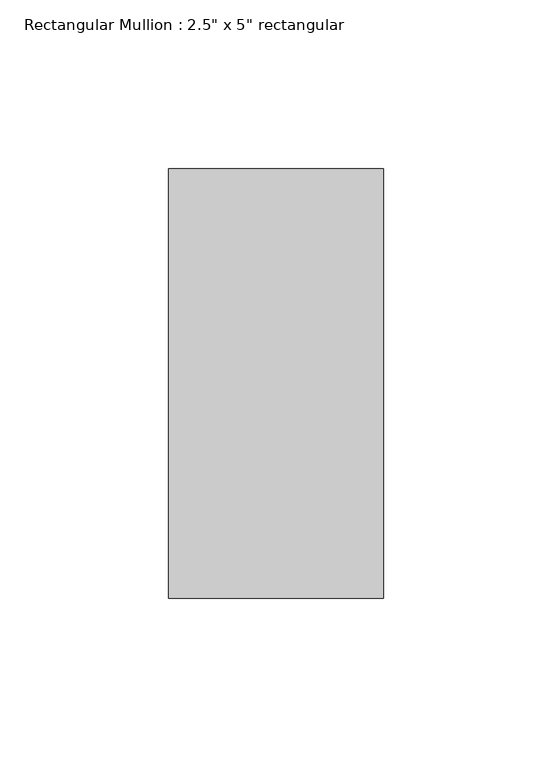
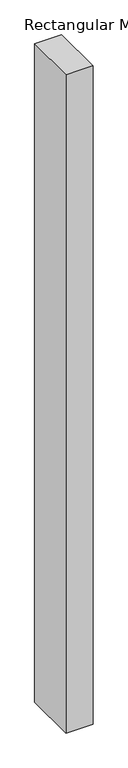
"""IFC4 building model written with IfcOpenShell, lengths in millimetres: member geometry."""

from ifc_helpers import new_model, si_unit, frame, origin, place, context, project, spatial, polyline, outline, extrude, source, transform, mapped, element, save


def member_ce46b7cd(model_context):
    return source(origin(), model_context, "Body", "SweptSolid", [
        extrude(outline(polyline([(0.0, 63.5), (0.0, -63.5), (-63.5, -63.5), (-63.5, 63.5), (0.0, 63.5)])), frame((0.0, 0.0, -1633.9367938), z_axis=(0.0, 0.0, 1.0), x_axis=(1.0, 0.0, 0.0)), (0.0, 0.0, 1.0), 1633.9367938),
    ])


if __name__ == "__main__":
    model = new_model("IFC4")
    model_context = context("Model", 3, world=origin())
    ifc_project = project(units=[si_unit("LENGTHUNIT", "METRE", prefix="MILLI")], contexts=[model_context])
    site = spatial("IfcSite", under=ifc_project)
    building = spatial("IfcBuilding", under=site)
    placement = place(None, origin())
    member_shape = member_ce46b7cd(model_context)
    element("IfcMember", 1, ObjectType="Rectangular Mullion : 2.5\" x 5\" rectangular", at=placement, inside=building, context=model_context, shape_type="MappedRepresentation", body=[
        mapped(member_shape, transform((0.0, 0.0, 0.0), x_axis=(1.0, 0.0, 0.0), y_axis=(0.0, 1.0, 0.0), z_axis=(0.0, 0.0, 1.0))),
    ])
    save(model, "model.ifc")

# Revit data of these elements
# Type "Rectangular Mullion : 2.5\" x 5\" rectangular"
#   built-in parameter 1007304 = 0.416667 (stored number, unit not read)
#   built-in parameter 1007301 = 0.104167 (stored number, unit not read)
#   built-in parameter 1007300 = 0.104167 (stored number, unit not read)
# Element 1 (IfcMember, "Rectangular Mullion : 2.5\" x 5\" rectangular")
#   Materials on its faces: "Aluminum"
# Materials
#   "Aluminum": class "Metal", colour RGB 247 247 247, transparency 0, Description = "Aluminum 6061", Cost = 0
